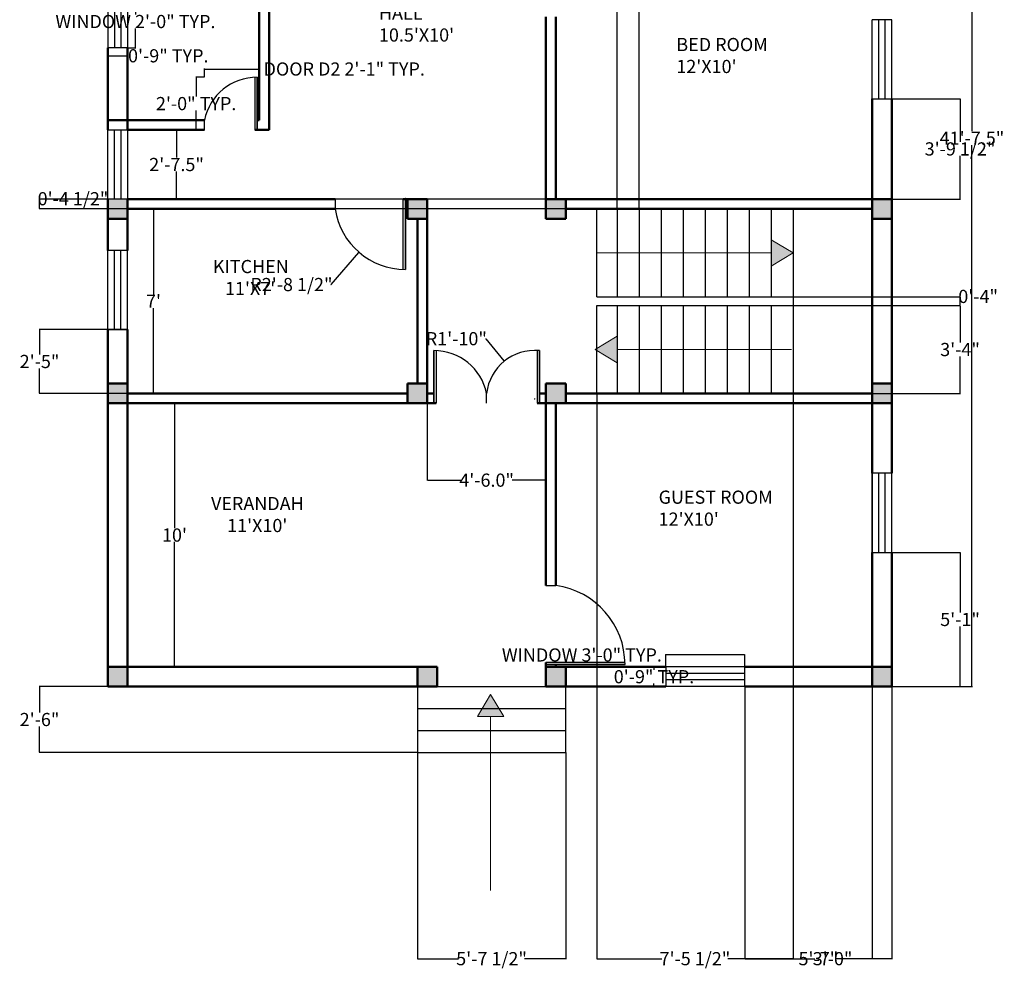
# Model space of a CAD drawing. Units: inches. Extents: x 1935 to 2390, y 6777 to 7449.
# Tile 1 of 2: x 1942 to 2390, y 6777 to 7213. Entities that reach past the tile are written whole.
import ezdxf

# ---------------------------------------------------------------- set-up
doc = ezdxf.new("R2010")
doc.units = ezdxf.units.IN
doc.header["$MEASUREMENT"] = 0
for name, color, linetype, lineweight in [('A-ANNO-DIMS', 7, 'Continuous', 18), ('A-ANNO-SYMB', 12, 'Continuous', 18), ('A-AREA-IDEN', 7, 'Continuous', 25), ('A-COLS', 42, 'Continuous', 50), ('A-COLS-PATT', 7, 'Continuous', 13), ('A-DOOR', 50, 'Continuous', 25), ('A-FLOR-STRS', 200, 'Continuous', 25), ('A-GLAZ', 140, 'Continuous', 25), ('A-WALL', 42, 'Continuous', 50)]:
    doc.layers.add(name, color=color, linetype=linetype, lineweight=lineweight)
doc.styles.get("Standard").update_dxf_attribs({"font": 'arial.ttf'})
doc.dimstyles.get("Standard").update_dxf_attribs({"dimtxt": 6, "dimasz": 0.18, "dimexe": 0.18, "dimexo": 0.0625, "dimgap": 0.09, "dimtad": 0, "dimtih": 1, "dimtoh": 1, "dimdec": 1, "dimzin": 0, "dimdsep": 46, "dimlunit": 3, "dimtxsty": 'Standard', "dimcen": 0.09, "dimclrd": 200, "dimclre": 200, "dimclrt": 200, "dimadec": 0, "dimazin": 0, "dimtfac": 1, "dimtdec": 1, "dimtofl": 0, "dimtmove": 0, "dimatfit": 3, "dimfxl": 1, "dimtolj": 1, "dimtzin": 0, "dimarcsym": 0})

# ---------------------------------------------------------------- blocks, each defined once
blk = doc.blocks.new('*D3')
at = {"layer": 'A-ANNO-DIMS', "color": 0, "lineweight": -2, "transparency": 16777216}
for p, q in [((1990.93, 7163.21), (2013.38, 7163.21)), ((2013.2, 7163.03), (2013.2, 7150.62)), ((2013.2, 7131.89), (2013.2, 7144.31)), ((1990.93, 7131.71), (2013.38, 7131.71))]:
    blk.add_line(p, q, dxfattribs=at)
at = {"layer": 'A-ANNO-DIMS', "color": 0, "transparency": 16777216}
for points in [[(2013.17, 7163.03), (2013.23, 7163.03), (2013.2, 7163.21)], [(2013.17, 7131.89), (2013.23, 7131.89), (2013.2, 7131.71)]]:
    blk.add_solid(points, dxfattribs=at)
at = {"layer": 'Defpoints', "color": 0, "transparency": 16777216}
for p in [(1990.87, 7163.21), (2013.2, 7163.21), (1990.87, 7131.71)]:
    blk.add_point(p, dxfattribs=at)
at = {"layer": 'A-ANNO-DIMS', "color": 0, "transparency": 16777216, "insert": (2013.2, 7147.46), "char_height": 6, "attachment_point": 5}
blk.add_mtext('\\A1;2\'-7.5"', dxfattribs=at)
blk = doc.blocks.new('*D4')
at = {"layer": 'A-ANNO-DIMS', "color": 0, "lineweight": -2, "transparency": 16777216}
for p, q in [((1990.93, 7127.21), (2002.86, 7127.21)), ((2002.68, 7127.03), (2002.68, 7088.3)), ((2002.68, 7043.39), (2002.68, 7082.12)), ((1990.93, 7043.21), (2002.86, 7043.21))]:
    blk.add_line(p, q, dxfattribs=at)
at = {"layer": 'A-ANNO-DIMS', "color": 0, "transparency": 16777216}
for points in [[(2002.65, 7127.03), (2002.71, 7127.03), (2002.68, 7127.21)], [(2002.65, 7043.39), (2002.71, 7043.39), (2002.68, 7043.21)]]:
    blk.add_solid(points, dxfattribs=at)
at = {"layer": 'Defpoints', "color": 0, "transparency": 16777216}
for p in [(1990.87, 7127.21), (1990.87, 7043.21), (2002.68, 7043.21)]:
    blk.add_point(p, dxfattribs=at)
at = {"layer": 'A-ANNO-DIMS', "color": 0, "transparency": 16777216, "insert": (2002.68, 7085.21), "char_height": 6, "attachment_point": 5}
blk.add_mtext("\\A1;7'", dxfattribs=at)
blk = doc.blocks.new('*D5')
at = {"layer": 'A-ANNO-DIMS', "color": 0, "lineweight": -2, "transparency": 16777216}
for p, q in [((1990.93, 7038.71), (2012.43, 7038.71)), ((2012.25, 7038.53), (2012.25, 6981.87)), ((2012.25, 6918.89), (2012.25, 6975.56)), ((1990.93, 6918.71), (2012.43, 6918.71))]:
    blk.add_line(p, q, dxfattribs=at)
at = {"layer": 'A-ANNO-DIMS', "color": 0, "transparency": 16777216}
for points in [[(2012.22, 7038.53), (2012.28, 7038.53), (2012.25, 7038.71)], [(2012.22, 6918.89), (2012.28, 6918.89), (2012.25, 6918.71)]]:
    blk.add_solid(points, dxfattribs=at)
at = {"layer": 'Defpoints', "color": 0, "transparency": 16777216}
for p in [(1990.87, 7038.71), (1990.87, 6918.71), (2012.25, 6918.71)]:
    blk.add_point(p, dxfattribs=at)
at = {"layer": 'A-ANNO-DIMS', "color": 0, "transparency": 16777216, "insert": (2012.25, 6978.71), "char_height": 6, "attachment_point": 5}
blk.add_mtext("\\A1;10'", dxfattribs=at)
blk = doc.blocks.new('*D6')
at = {"layer": 'A-ANNO-DIMS', "color": 0, "lineweight": -2, "transparency": 16777216}
for p, q in [((2127.37, 7038.65), (2127.37, 7003.54)), ((2181.37, 7038.65), (2181.37, 7003.54)), ((2127.55, 7003.72), (2142.68, 7003.72)), ((2181.19, 7003.72), (2166.05, 7003.72))]:
    blk.add_line(p, q, dxfattribs=at)
at = {"layer": 'A-ANNO-DIMS', "color": 0, "transparency": 16777216}
for points in [[(2127.55, 7003.75), (2127.55, 7003.69), (2127.37, 7003.72)], [(2181.19, 7003.75), (2181.19, 7003.69), (2181.37, 7003.72)]]:
    blk.add_solid(points, dxfattribs=at)
at = {"layer": 'Defpoints', "color": 0, "transparency": 16777216}
for p in [(2127.37, 7038.71), (2181.37, 7038.71), (2181.37, 7003.72)]:
    blk.add_point(p, dxfattribs=at)
at = {"layer": 'A-ANNO-DIMS', "color": 0, "transparency": 16777216, "insert": (2154.37, 7003.72), "char_height": 6, "attachment_point": 5}
blk.add_mtext('\\A1;4\'-6.0"', dxfattribs=at)
blk = doc.blocks.new('*D9')
at = {"layer": 'A-ANNO-DIMS', "color": 0, "lineweight": -2, "transparency": 16777216}
for p, q in [((2338.93, 7409.21), (2375.52, 7409.21)), ((2375.34, 7409.03), (2375.34, 7162.62)), ((2375.34, 6909.89), (2375.34, 7156.31)), ((2338.93, 6909.71), (2375.52, 6909.71))]:
    blk.add_line(p, q, dxfattribs=at)
at = {"layer": 'A-ANNO-DIMS', "color": 0, "transparency": 16777216}
for points in [[(2375.31, 7409.03), (2375.37, 7409.03), (2375.34, 7409.21)], [(2375.31, 6909.89), (2375.37, 6909.89), (2375.34, 6909.71)]]:
    blk.add_solid(points, dxfattribs=at)
at = {"layer": 'Defpoints', "color": 0, "transparency": 16777216}
for p in [(2338.87, 7409.21), (2338.87, 6909.71), (2375.34, 6909.71)]:
    blk.add_point(p, dxfattribs=at)
at = {"layer": 'A-ANNO-DIMS', "color": 0, "transparency": 16777216, "insert": (2375.34, 7159.46), "char_height": 6, "attachment_point": 5}
blk.add_mtext('\\A1;41\'-7.5"', dxfattribs=at)
blk = doc.blocks.new('WIN-36IN')
for p, q in [((0, 9), (0, 0)), ((0, 9), (36, 9)), ((36, 0), (36, 9)), ((0, 6), (36, 6)), ((0, 3), (36, 3)), ((0, 0), (36, 0))]:
    blk.add_line(p, q)
blk = doc.blocks.new('WIN-24IN')
for p, q in [((0, 24), (9, 24)), ((0, 24), (0, 0)), ((3, 24), (3, 0)), ((6, 24), (6, 0)), ((9, 24), (9, 0)), ((9, 0), (0, 0))]:
    blk.add_line(p, q)
blk = doc.blocks.new('DOOR-SINGLE-36IN')
for p, q in [((0, 37), (4.5, 37)), ((0, 1), (0, 2)), ((36, 2), (0, 2)), ((0, 0), (0, 1)), ((0, 1), (36, 1)), ((36, 1), (0, 1))]:
    blk.add_line(p, q)
blk.add_arc((-0.32, 1), 36.32, 0, 82.3719)
blk = doc.blocks.new('DOOR-SINGLE-24IN')
for p, q in [((23, 24), (23, 0)), ((24, 0), (24, 24)), ((24, 24), (24, 0)), ((0, 0), (0, 4.5)), ((24, 0), (23, 0)), ((25, 0), (24, 0))]:
    blk.add_line(p, q)
blk.add_arc((24, -0.52), 24.52, 90, 168.1877)
blk = doc.blocks.new('STAIR-DIRECTION')
h = blk.add_hatch(color=256)
h.dxf.hatch_style = 1
h.paths.add_polyline_path([(79.31, 12), (79.31, 0), (89.31, 6)])
for p, q in [((79.31, 12), (79.31, 0)), ((89.31, 6), (79.31, 12)), ((0, 6), (79.31, 6)), ((79.31, 0), (89.31, 6))]:
    blk.add_line(p, q)
blk = doc.blocks.new('*D16')
at = {"layer": 'A-ANNO-DIMS', "color": 200, "lineweight": -2, "transparency": 16777216}
for p, q in [((2235.96, 6924.11), (2235.78, 6924.11)), ((2235.96, 6918.78), (2235.96, 6924.29)), ((2271.78, 6924.11), (2236.14, 6924.11)), ((2271.96, 6918.78), (2271.96, 6924.29))]:
    blk.add_line(p, q, dxfattribs=at)
at = {"layer": 'A-ANNO-DIMS', "color": 200, "transparency": 16777216}
for points in [[(2236.14, 6924.14), (2236.14, 6924.08), (2235.96, 6924.11)], [(2271.78, 6924.14), (2271.78, 6924.08), (2271.96, 6924.11)]]:
    blk.add_solid(points, dxfattribs=at)
at = {"layer": 'Defpoints', "color": 0, "transparency": 16777216}
for p in [(2235.96, 6924.11), (2235.96, 6918.71), (2271.96, 6918.71)]:
    blk.add_point(p, dxfattribs=at)
at = {"layer": 'A-ANNO-DIMS', "color": 200, "transparency": 16777216, "insert": (2197.73, 6924.11), "char_height": 6, "attachment_point": 5}
blk.add_mtext('\\A1;WINDOW 3\'-0" TYP.', dxfattribs=at)
blk = doc.blocks.new('*D17')
at = {"layer": 'A-ANNO-DIMS', "color": 200, "lineweight": -2, "transparency": 16777216}
for p, q in [((2235.9, 6918.71), (2230.38, 6918.71)), ((2230.56, 6918.53), (2230.56, 6917.37)), ((2235.9, 6909.71), (2230.38, 6909.71)), ((2230.56, 6909.89), (2230.56, 6911.06))]:
    blk.add_line(p, q, dxfattribs=at)
at = {"layer": 'A-ANNO-DIMS', "color": 200, "transparency": 16777216}
for points in [[(2230.53, 6918.53), (2230.59, 6918.53), (2230.56, 6918.71)], [(2230.53, 6909.89), (2230.59, 6909.89), (2230.56, 6909.71)]]:
    blk.add_solid(points, dxfattribs=at)
at = {"layer": 'Defpoints', "color": 0, "transparency": 16777216}
for p in [(2235.96, 6918.71), (2230.56, 6909.71), (2235.96, 6909.71)]:
    blk.add_point(p, dxfattribs=at)
at = {"layer": 'A-ANNO-DIMS', "color": 200, "transparency": 16777216, "insert": (2230.56, 6914.21), "char_height": 6, "attachment_point": 5}
blk.add_mtext('\\A1;0\'-9" TYP.', dxfattribs=at)
blk = doc.blocks.new('*D18')
at = {"layer": 'A-ANNO-DIMS', "color": 200, "lineweight": -2, "transparency": 16777216}
for p, q in [((1990.93, 7224.58), (1994.65, 7224.58)), ((1994.47, 7224.4), (1994.47, 7215.77)), ((1994.47, 7200.76), (1994.47, 7209.39)), ((1990.93, 7200.58), (1994.65, 7200.58))]:
    blk.add_line(p, q, dxfattribs=at)
at = {"layer": 'A-ANNO-DIMS', "color": 200, "transparency": 16777216}
for points in [[(1994.44, 7224.4), (1994.5, 7224.4), (1994.47, 7224.58)], [(1994.44, 7200.76), (1994.5, 7200.76), (1994.47, 7200.58)]]:
    blk.add_solid(points, dxfattribs=at)
at = {"layer": 'Defpoints', "color": 0, "transparency": 16777216}
for p in [(1990.87, 7224.58), (1994.47, 7224.58), (1990.87, 7200.58)]:
    blk.add_point(p, dxfattribs=at)
at = {"layer": 'A-ANNO-DIMS', "color": 200, "transparency": 16777216, "insert": (1994.47, 7212.58), "char_height": 6, "attachment_point": 5}
blk.add_mtext('\\A1;WINDOW 2\'-0" TYP.', dxfattribs=at)
blk = doc.blocks.new('*D19')
at = {"layer": 'A-ANNO-DIMS', "color": 200, "lineweight": -2, "transparency": 16777216}
for p, q in [((1981.87, 7200.52), (1981.87, 7196.8)), ((1990.87, 7200.52), (1990.87, 7196.8)), ((1982.05, 7196.98), (1990.69, 7196.98)), ((1990.87, 7196.98), (1991.05, 7196.98))]:
    blk.add_line(p, q, dxfattribs=at)
at = {"layer": 'A-ANNO-DIMS', "color": 200, "transparency": 16777216}
for points in [[(1982.05, 7197.01), (1982.05, 7196.95), (1981.87, 7196.98)], [(1990.69, 7197.01), (1990.69, 7196.95), (1990.87, 7196.98)]]:
    blk.add_solid(points, dxfattribs=at)
at = {"layer": 'Defpoints', "color": 0, "transparency": 16777216}
for p in [(1981.87, 7200.58), (1990.87, 7200.58), (1990.87, 7196.98)]:
    blk.add_point(p, dxfattribs=at)
at = {"layer": 'A-ANNO-DIMS', "color": 200, "transparency": 16777216, "insert": (2009.42, 7196.98), "char_height": 6, "attachment_point": 5}
blk.add_mtext('\\A1;0\'-9" TYP.', dxfattribs=at)
blk = doc.blocks.new('*D22')
at = {"layer": 'A-ANNO-DIMS', "color": 200, "lineweight": -2, "transparency": 16777216}
for p, q in [((2025.87, 7187.28), (2025.87, 7191.14)), ((2026.05, 7190.96), (2050.69, 7190.96)), ((2050.87, 7187.28), (2050.87, 7191.14)), ((2050.87, 7190.96), (2051.05, 7190.96))]:
    blk.add_line(p, q, dxfattribs=at)
at = {"layer": 'A-ANNO-DIMS', "color": 200, "transparency": 16777216}
for points in [[(2026.05, 7190.99), (2026.05, 7190.93), (2025.87, 7190.96)], [(2050.69, 7190.99), (2050.69, 7190.93), (2050.87, 7190.96)]]:
    blk.add_solid(points, dxfattribs=at)
at = {"layer": 'Defpoints', "color": 0, "transparency": 16777216}
for p in [(2050.87, 7190.96), (2025.87, 7187.21), (2050.87, 7187.21)]:
    blk.add_point(p, dxfattribs=at)
at = {"layer": 'A-ANNO-DIMS', "color": 200, "transparency": 16777216, "insert": (2089.53, 7190.96), "char_height": 6, "attachment_point": 5}
blk.add_mtext('\\A1;DOOR D2 2\'-1" TYP.', dxfattribs=at)
blk = doc.blocks.new('*D23')
at = {"layer": 'A-ANNO-DIMS', "color": 200, "lineweight": -2, "transparency": 16777216}
for p, q in [((2025.8, 7187.21), (2021.94, 7187.21)), ((2022.12, 7187.03), (2022.12, 7178.37)), ((2022.12, 7163.39), (2022.12, 7172.06)), ((2025.8, 7163.21), (2021.94, 7163.21))]:
    blk.add_line(p, q, dxfattribs=at)
at = {"layer": 'A-ANNO-DIMS', "color": 200, "transparency": 16777216}
for points in [[(2022.09, 7187.03), (2022.15, 7187.03), (2022.12, 7187.21)], [(2022.09, 7163.39), (2022.15, 7163.39), (2022.12, 7163.21)]]:
    blk.add_solid(points, dxfattribs=at)
at = {"layer": 'Defpoints', "color": 0, "transparency": 16777216}
for p in [(2022.12, 7187.21), (2025.87, 7187.21), (2025.87, 7163.21)]:
    blk.add_point(p, dxfattribs=at)
at = {"layer": 'A-ANNO-DIMS', "color": 200, "transparency": 16777216, "insert": (2022.12, 7175.21), "char_height": 6, "attachment_point": 5}
blk.add_mtext('\\A1;2\'-0" TYP.', dxfattribs=at)
blk = doc.blocks.new('*D24')
at = {"layer": 'A-ANNO-DIMS', "color": 200, "lineweight": -2, "transparency": 16777216}
for p, q in [((2122.87, 6879.65), (2122.87, 6785.62)), ((2190.37, 6879.65), (2190.37, 6785.62)), ((2123.05, 6785.8), (2141.56, 6785.8)), ((2190.19, 6785.8), (2171.67, 6785.8))]:
    blk.add_line(p, q, dxfattribs=at)
at = {"layer": 'A-ANNO-DIMS', "color": 200, "transparency": 16777216}
for points in [[(2123.05, 6785.83), (2123.05, 6785.77), (2122.87, 6785.8)], [(2190.19, 6785.83), (2190.19, 6785.77), (2190.37, 6785.8)]]:
    blk.add_solid(points, dxfattribs=at)
at = {"layer": 'Defpoints', "color": 0, "transparency": 16777216}
for p in [(2122.87, 6879.71), (2190.37, 6879.71), (2190.37, 6785.8)]:
    blk.add_point(p, dxfattribs=at)
at = {"layer": 'A-ANNO-DIMS', "color": 200, "transparency": 16777216, "insert": (2156.62, 6785.8), "char_height": 6, "attachment_point": 5}
blk.add_mtext('\\A1;5\'-7 1/2"', dxfattribs=at)
blk = doc.blocks.new('*D25')
at = {"layer": 'A-ANNO-DIMS', "color": 200, "lineweight": -2, "transparency": 16777216}
for p, q in [((2122.8, 6909.71), (1950.64, 6909.71)), ((1950.82, 6909.53), (1950.82, 6897.87)), ((1950.82, 6879.89), (1950.82, 6891.56)), ((2122.8, 6879.71), (1950.64, 6879.71))]:
    blk.add_line(p, q, dxfattribs=at)
at = {"layer": 'A-ANNO-DIMS', "color": 200, "transparency": 16777216}
for points in [[(1950.79, 6909.53), (1950.85, 6909.53), (1950.82, 6909.71)], [(1950.79, 6879.89), (1950.85, 6879.89), (1950.82, 6879.71)]]:
    blk.add_solid(points, dxfattribs=at)
at = {"layer": 'Defpoints', "color": 0, "transparency": 16777216}
for p in [(1950.82, 6909.71), (2122.87, 6909.71), (2122.87, 6879.71)]:
    blk.add_point(p, dxfattribs=at)
at = {"layer": 'A-ANNO-DIMS', "color": 200, "transparency": 16777216, "insert": (1950.82, 6894.71), "char_height": 6, "attachment_point": 5}
blk.add_mtext('\\A1;2\'-6"', dxfattribs=at)
blk = doc.blocks.new('*D26')
at = {"layer": 'A-ANNO-DIMS', "color": 200, "lineweight": -2, "transparency": 16777216}
for p, q in [((2204.56, 7043.15), (2204.56, 6785.62)), ((2293.87, 7043.15), (2293.87, 6785.62)), ((2204.74, 6785.8), (2234.18, 6785.8)), ((2293.69, 6785.8), (2264.24, 6785.8))]:
    blk.add_line(p, q, dxfattribs=at)
at = {"layer": 'A-ANNO-DIMS', "color": 200, "transparency": 16777216}
for points in [[(2204.74, 6785.83), (2204.74, 6785.77), (2204.56, 6785.8)], [(2293.69, 6785.83), (2293.69, 6785.77), (2293.87, 6785.8)]]:
    blk.add_solid(points, dxfattribs=at)
at = {"layer": 'Defpoints', "color": 0, "transparency": 16777216}
for p in [(2204.56, 7043.21), (2293.87, 7043.21), (2293.87, 6785.8)]:
    blk.add_point(p, dxfattribs=at)
at = {"layer": 'A-ANNO-DIMS', "color": 200, "transparency": 16777216, "insert": (2249.21, 6785.8), "char_height": 6, "attachment_point": 5}
blk.add_mtext('\\A1;7\'-5 1/2"', dxfattribs=at)
blk = doc.blocks.new('*D27')
at = {"layer": 'A-ANNO-DIMS', "color": 200, "lineweight": -2, "transparency": 16777216}
for p, q in [((2293.93, 7083.21), (2370.1, 7083.21)), ((2369.92, 7083.03), (2369.92, 7066.37)), ((2369.92, 7043.39), (2369.92, 7060.06)), ((2293.93, 7043.21), (2370.1, 7043.21))]:
    blk.add_line(p, q, dxfattribs=at)
at = {"layer": 'A-ANNO-DIMS', "color": 200, "transparency": 16777216}
for points in [[(2369.89, 7083.03), (2369.95, 7083.03), (2369.92, 7083.21)], [(2369.89, 7043.39), (2369.95, 7043.39), (2369.92, 7043.21)]]:
    blk.add_solid(points, dxfattribs=at)
at = {"layer": 'Defpoints', "color": 0, "transparency": 16777216}
for p in [(2293.87, 7083.21), (2369.92, 7083.21), (2293.87, 7043.21)]:
    blk.add_point(p, dxfattribs=at)
at = {"layer": 'A-ANNO-DIMS', "color": 200, "transparency": 16777216, "insert": (2369.92, 7063.21), "char_height": 6, "attachment_point": 5}
blk.add_mtext('\\A1;3\'-4"', dxfattribs=at)
blk = doc.blocks.new('*D28')
at = {"layer": 'A-ANNO-DIMS', "color": 200, "lineweight": -2, "transparency": 16777216}
for p, q in [((2293.93, 7087.21), (2370.1, 7087.21)), ((2293.93, 7083.21), (2370.1, 7083.21)), ((2369.92, 7087.21), (2369.92, 7087.39)), ((2369.92, 7087.39), (2370.1, 7087.39)), ((2369.92, 7083.39), (2369.92, 7087.03))]:
    blk.add_line(p, q, dxfattribs=at)
at = {"layer": 'A-ANNO-DIMS', "color": 200, "transparency": 16777216}
for points in [[(2369.89, 7087.03), (2369.95, 7087.03), (2369.92, 7087.21)], [(2369.89, 7083.39), (2369.95, 7083.39), (2369.92, 7083.21)]]:
    blk.add_solid(points, dxfattribs=at)
at = {"layer": 'Defpoints', "color": 0, "transparency": 16777216}
for p in [(2293.87, 7087.21), (2293.87, 7083.21), (2369.92, 7087.21)]:
    blk.add_point(p, dxfattribs=at)
at = {"layer": 'A-ANNO-DIMS', "color": 200, "transparency": 16777216, "insert": (2378.16, 7087.39), "char_height": 6, "attachment_point": 5}
blk.add_mtext('\\A1;0\'-4"', dxfattribs=at)
blk = doc.blocks.new('*D29')
at = {"layer": 'A-ANNO-DIMS', "color": 200, "lineweight": -2, "transparency": 16777216}
for p, q in [((2293.87, 7043.15), (2293.87, 6785.62)), ((2329.87, 7043.15), (2329.87, 6785.62)), ((2294.05, 6785.8), (2303.8, 6785.8)), ((2329.69, 6785.8), (2319.93, 6785.8))]:
    blk.add_line(p, q, dxfattribs=at)
at = {"layer": 'A-ANNO-DIMS', "color": 200, "transparency": 16777216}
for points in [[(2294.05, 6785.83), (2294.05, 6785.77), (2293.87, 6785.8)], [(2329.69, 6785.83), (2329.69, 6785.77), (2329.87, 6785.8)]]:
    blk.add_solid(points, dxfattribs=at)
at = {"layer": 'Defpoints', "color": 0, "transparency": 16777216}
for p in [(2293.87, 7043.21), (2329.87, 7043.21), (2329.87, 6785.8)]:
    blk.add_point(p, dxfattribs=at)
at = {"layer": 'A-ANNO-DIMS', "color": 200, "transparency": 16777216, "insert": (2311.87, 6785.8), "char_height": 6, "attachment_point": 5}
blk.add_mtext('\\A1;3\'-0"', dxfattribs=at)
blk = doc.blocks.new('*D30')
at = {"layer": 'A-ANNO-DIMS', "color": 200, "lineweight": -2, "transparency": 16777216}
for p, q in [((2213.87, 7127.28), (2213.87, 7440.44)), ((2214.05, 7440.26), (2223.69, 7440.26)), ((2223.87, 7127.28), (2223.87, 7440.44)), ((2223.87, 7440.26), (2224.05, 7440.26))]:
    blk.add_line(p, q, dxfattribs=at)
at = {"layer": 'A-ANNO-DIMS', "color": 200, "transparency": 16777216}
for points in [[(2214.05, 7440.29), (2214.05, 7440.23), (2213.87, 7440.26)], [(2223.69, 7440.29), (2223.69, 7440.23), (2223.87, 7440.26)]]:
    blk.add_solid(points, dxfattribs=at)
at = {"layer": 'Defpoints', "color": 0, "transparency": 16777216}
for p in [(2223.87, 7440.26), (2213.87, 7127.21), (2223.87, 7127.21)]:
    blk.add_point(p, dxfattribs=at)
at = {"layer": 'A-ANNO-DIMS', "color": 200, "transparency": 16777216, "insert": (2234.44, 7440.26), "char_height": 6, "attachment_point": 5}
blk.add_mtext('\\A1;0\'-10"', dxfattribs=at)
blk = doc.blocks.new('*D31')
at = {"layer": 'A-ANNO-DIMS', "color": 200, "lineweight": -2, "transparency": 16777216}
for p, q in [((2181.3, 7131.71), (1950.64, 7131.71)), ((1950.82, 7131.71), (1950.82, 7131.89)), ((1950.82, 7131.89), (1951, 7131.89)), ((1950.82, 7127.39), (1950.82, 7131.53)), ((2190.3, 7127.21), (1950.64, 7127.21))]:
    blk.add_line(p, q, dxfattribs=at)
at = {"layer": 'A-ANNO-DIMS', "color": 200, "transparency": 16777216}
for points in [[(1950.79, 7131.53), (1950.85, 7131.53), (1950.82, 7131.71)], [(1950.79, 7127.39), (1950.85, 7127.39), (1950.82, 7127.21)]]:
    blk.add_solid(points, dxfattribs=at)
at = {"layer": 'Defpoints', "color": 0, "transparency": 16777216}
for p in [(1950.82, 7131.71), (2181.37, 7131.71), (2190.37, 7127.21)]:
    blk.add_point(p, dxfattribs=at)
at = {"layer": 'A-ANNO-DIMS', "color": 200, "transparency": 16777216, "insert": (1966.05, 7131.89), "char_height": 6, "attachment_point": 5}
blk.add_mtext('\\A1;0\'-4 1/2"', dxfattribs=at)
blk = doc.blocks.new('*D36')
at = {"layer": 'A-ANNO-DIMS', "color": 200, "lineweight": -2, "transparency": 16777216}
for p, q in [((2329.93, 7177.42), (2370.1, 7177.42)), ((2369.92, 7177.24), (2369.92, 7157.76)), ((2369.92, 7131.89), (2369.92, 7151.37)), ((2329.93, 7131.71), (2370.1, 7131.71))]:
    blk.add_line(p, q, dxfattribs=at)
at = {"layer": 'A-ANNO-DIMS', "color": 200, "transparency": 16777216}
for points in [[(2369.89, 7177.24), (2369.95, 7177.24), (2369.92, 7177.42)], [(2369.89, 7131.89), (2369.95, 7131.89), (2369.92, 7131.71)]]:
    blk.add_solid(points, dxfattribs=at)
at = {"layer": 'Defpoints', "color": 0, "transparency": 16777216}
for p in [(2329.87, 7177.42), (2369.92, 7177.42), (2329.87, 7131.71)]:
    blk.add_point(p, dxfattribs=at)
at = {"layer": 'A-ANNO-DIMS', "color": 200, "transparency": 16777216, "insert": (2369.92, 7154.57), "char_height": 6, "attachment_point": 5}
blk.add_mtext('\\A1;3\'-9 1/2"', dxfattribs=at)
blk = doc.blocks.new('*D37')
at = {"layer": 'A-ANNO-DIMS', "color": 200, "lineweight": -2, "transparency": 16777216}
for p, q in [((2338.93, 6970.84), (2370.1, 6970.84)), ((2369.92, 6970.66), (2369.92, 6943.43)), ((2369.92, 6909.89), (2369.92, 6937.12)), ((2338.93, 6909.71), (2370.1, 6909.71))]:
    blk.add_line(p, q, dxfattribs=at)
at = {"layer": 'A-ANNO-DIMS', "color": 200, "transparency": 16777216}
for points in [[(2369.89, 6970.66), (2369.95, 6970.66), (2369.92, 6970.84)], [(2369.89, 6909.89), (2369.95, 6909.89), (2369.92, 6909.71)]]:
    blk.add_solid(points, dxfattribs=at)
at = {"layer": 'Defpoints', "color": 0, "transparency": 16777216}
for p in [(2338.87, 6970.84), (2369.92, 6970.84), (2338.87, 6909.71)]:
    blk.add_point(p, dxfattribs=at)
at = {"layer": 'A-ANNO-DIMS', "color": 200, "transparency": 16777216, "insert": (2369.92, 6940.28), "char_height": 6, "attachment_point": 5}
blk.add_mtext('\\A1;5\'-1"', dxfattribs=at)
blk = doc.blocks.new('*D38')
at = {"layer": 'A-ANNO-DIMS', "color": 200, "lineweight": -2, "transparency": 16777216}
for p, q in [((2271.96, 6909.65), (2271.96, 6785.62)), ((2338.87, 6909.65), (2338.87, 6785.62)), ((2272.14, 6785.8), (2297.35, 6785.8)), ((2338.69, 6785.8), (2313.48, 6785.8))]:
    blk.add_line(p, q, dxfattribs=at)
at = {"layer": 'A-ANNO-DIMS', "color": 200, "transparency": 16777216}
for points in [[(2272.14, 6785.83), (2272.14, 6785.77), (2271.96, 6785.8)], [(2338.69, 6785.83), (2338.69, 6785.77), (2338.87, 6785.8)]]:
    blk.add_solid(points, dxfattribs=at)
at = {"layer": 'Defpoints', "color": 0, "transparency": 16777216}
for p in [(2271.96, 6909.71), (2338.87, 6909.71), (2338.87, 6785.8)]:
    blk.add_point(p, dxfattribs=at)
at = {"layer": 'A-ANNO-DIMS', "color": 200, "transparency": 16777216, "insert": (2305.41, 6785.8), "char_height": 6, "attachment_point": 5}
blk.add_mtext('\\A1;5\'-7"', dxfattribs=at)
blk = doc.blocks.new('*D41')
at = {"layer": 'A-ANNO-DIMS', "color": 200, "lineweight": -2, "transparency": 16777216}
for p, q in [((1990.8, 7072.32), (1950.64, 7072.32)), ((1950.82, 7072.14), (1950.82, 7060.92)), ((1950.82, 7043.39), (1950.82, 7054.62)), ((1990.8, 7043.21), (1950.64, 7043.21))]:
    blk.add_line(p, q, dxfattribs=at)
at = {"layer": 'A-ANNO-DIMS', "color": 200, "transparency": 16777216}
for points in [[(1950.79, 7072.14), (1950.85, 7072.14), (1950.82, 7072.32)], [(1950.79, 7043.39), (1950.85, 7043.39), (1950.82, 7043.21)]]:
    blk.add_solid(points, dxfattribs=at)
at = {"layer": 'Defpoints', "color": 0, "transparency": 16777216}
for p in [(1950.82, 7072.32), (1990.87, 7072.32), (1990.87, 7043.21)]:
    blk.add_point(p, dxfattribs=at)
at = {"layer": 'A-ANNO-DIMS', "color": 200, "transparency": 16777216, "insert": (1950.82, 7057.77), "char_height": 6, "attachment_point": 5}
blk.add_mtext('\\A1;2\'-5"', dxfattribs=at)
blk = doc.blocks.new('*D43')
at = {"layer": 'A-ANNO-DIMS', "color": 200, "lineweight": -2, "transparency": 16777216}
for p, q in [((2117.28, 7132.08), (2117.46, 7132.08)), ((2117.37, 7131.99), (2117.37, 7132.17)), ((2083.61, 7092.8), (2096.15, 7107.4)), ((2083.43, 7092.8), (2083.61, 7092.8))]:
    blk.add_line(p, q, dxfattribs=at)
at = {"layer": 'A-ANNO-DIMS', "color": 200, "transparency": 16777216}
blk.add_solid([(2096.13, 7107.42), (2096.17, 7107.38), (2096.27, 7107.53)], dxfattribs=at)
at = {"layer": 'Defpoints', "color": 0, "transparency": 16777216}
for p in [(2117.37, 7132.08), (2096.27, 7107.53)]:
    blk.add_point(p, dxfattribs=at)
at = {"layer": 'A-ANNO-DIMS', "color": 200, "transparency": 16777216, "insert": (2065.5, 7092.8), "char_height": 6, "attachment_point": 5}
blk.add_mtext('\\A1;R2\'-8 1/2"', dxfattribs=at)
blk = doc.blocks.new('*D45')
at = {"layer": 'A-ANNO-DIMS', "color": 200, "lineweight": -2, "transparency": 16777216}
for p, q in [((2153.85, 7068.15), (2154.03, 7068.15)), ((2154.03, 7068.15), (2162.26, 7058.01)), ((2176.2, 7040.75), (2176.38, 7040.75)), ((2176.29, 7040.66), (2176.29, 7040.84))]:
    blk.add_line(p, q, dxfattribs=at)
at = {"layer": 'A-ANNO-DIMS', "color": 200, "transparency": 16777216}
blk.add_solid([(2162.29, 7058.03), (2162.24, 7057.99), (2162.38, 7057.87)], dxfattribs=at)
at = {"layer": 'Defpoints', "color": 0, "transparency": 16777216}
for p in [(2162.38, 7057.87), (2176.29, 7040.75)]:
    blk.add_point(p, dxfattribs=at)
at = {"layer": 'A-ANNO-DIMS', "color": 200, "transparency": 16777216, "insert": (2140.58, 7068.15), "char_height": 6, "attachment_point": 5}
blk.add_mtext('\\A1;R1\'-10"', dxfattribs=at)

msp = doc.modelspace()

# ---------------------------------------------------------------- hatches: boundary and pattern name
at = {"layer": 'A-COLS-PATT'}
h = msp.add_hatch(color=256, dxfattribs=at)
h.dxf.hatch_style = 1
h.paths.add_polyline_path([(1990.87, 7409.21), (1981.87, 7409.21), (1981.87, 7400.21), (1990.87, 7400.21)])
h.paths.add_polyline_path([(2127.37, 7409.21), (2118.37, 7409.21), (2118.37, 7400.21), (2127.37, 7400.21)])
h.paths.add_polyline_path([(2190.37, 7409.21), (2181.37, 7409.21), (2181.37, 7400.21), (2190.37, 7400.21)])
h.paths.add_polyline_path([(2338.87, 7409.21), (2329.87, 7409.21), (2329.87, 7400.21), (2338.87, 7400.21)])
h.paths.add_polyline_path([(1990.87, 7260.71), (1981.87, 7260.71), (1981.87, 7251.71), (1990.87, 7251.71)])
h.paths.add_polyline_path([(2127.37, 7260.71), (2118.37, 7260.71), (2118.37, 7251.71), (2127.37, 7251.71)])
h.paths.add_polyline_path([(2190.37, 7260.71), (2181.37, 7260.71), (2181.37, 7251.71), (2190.37, 7251.71)])
h.paths.add_polyline_path([(2338.87, 7260.71), (2329.87, 7260.71), (2329.87, 7251.71), (2338.87, 7251.71)])
h.paths.add_polyline_path([(1990.87, 7131.71), (1981.87, 7131.71), (1981.87, 7122.71), (1990.87, 7122.71)])
h.paths.add_polyline_path([(2127.37, 7131.71), (2118.37, 7131.71), (2118.37, 7122.71), (2127.37, 7122.71)])
h.paths.add_polyline_path([(1990.87, 7047.71), (1981.87, 7047.71), (1981.87, 7038.71), (1990.87, 7038.71)])
h.paths.add_polyline_path([(2127.37, 7047.71), (2118.37, 7047.71), (2118.37, 7038.71), (2127.37, 7038.71)])
h.paths.add_polyline_path([(1990.87, 6918.71), (1981.87, 6918.71), (1981.87, 6909.71), (1990.87, 6909.71)])
h.paths.add_polyline_path([(2131.87, 6918.71), (2122.87, 6918.71), (2122.87, 6909.71), (2131.87, 6909.71)])
h.paths.add_polyline_path([(2190.37, 6918.71), (2181.37, 6918.71), (2181.37, 6909.71), (2190.37, 6909.71)])
h.paths.add_polyline_path([(2338.87, 6918.71), (2329.87, 6918.71), (2329.87, 6909.71), (2338.87, 6909.71)])
h.paths.add_polyline_path([(2190.37, 7047.71), (2181.37, 7047.71), (2181.37, 7038.71), (2190.37, 7038.71)])
h.paths.add_polyline_path([(2338.87, 7047.71), (2329.87, 7047.71), (2329.87, 7038.71), (2338.87, 7038.71)])
h.paths.add_polyline_path([(2190.37, 7131.71), (2181.37, 7131.71), (2181.37, 7122.71), (2190.37, 7122.71)])
h.paths.add_polyline_path([(2338.87, 7131.71), (2329.87, 7131.71), (2329.87, 7122.71), (2338.87, 7122.71)])

# ---------------------------------------------------------------- linework, layer by layer
at = {"layer": 'A-ANNO-SYMB'}
msp.add_line((2283.87, 7107.21), (2283.87, 7113.21), dxfattribs=at)
at = {"layer": 'A-COLS'}
for p, q in [((1981.87, 7131.71), (1981.87, 7122.71)), ((2127.37, 7131.71), (2118.37, 7131.71)), ((2118.37, 7131.71), (2118.37, 7122.71)), ((2181.37, 7131.71), (2190.37, 7131.71)), ((2181.37, 7122.71), (2181.37, 7131.71)), ((2190.37, 7131.71), (2190.37, 7122.71)), ((2329.87, 7131.71), (2329.87, 7122.71)), ((1981.87, 7122.71), (1990.87, 7122.71)), ((2118.37, 7122.71), (2127.37, 7122.71)), ((2190.37, 7122.71), (2181.37, 7122.71)), ((2329.87, 7122.71), (2338.87, 7122.71)), ((1981.87, 7038.71), (1981.87, 7047.71)), ((1981.87, 7047.71), (1990.87, 7047.71)), ((2127.37, 7047.71), (2118.37, 7047.71)), ((2118.37, 7047.71), (2118.37, 7038.71)), ((2127.37, 7038.71), (2127.37, 7047.71)), ((2181.37, 7038.71), (2181.37, 7047.71)), ((2181.37, 7047.71), (2190.37, 7047.71)), ((2190.37, 7047.71), (2190.37, 7038.71)), ((2338.87, 7047.71), (2329.87, 7047.71)), ((2329.87, 7047.71), (2329.87, 7038.71)), ((2338.87, 7038.71), (2338.87, 7047.71)), ((1981.87, 6909.71), (1981.87, 6918.71)), ((2122.87, 6918.71), (2122.87, 6909.71)), ((2122.87, 6918.71), (2131.87, 6918.71)), ((2131.87, 6918.71), (2131.87, 6909.71)), ((2181.37, 6918.71), (2190.37, 6918.71)), ((2190.37, 6918.71), (2190.37, 6909.71))]:
    msp.add_line(p, q, dxfattribs=at)
at = {"layer": 'A-DOOR'}
for p, q in [((2085.37, 7131.71), (2085.37, 7127.21)), ((2117.37, 7131.71), (2116.37, 7131.71)), ((2116.37, 7099.71), (2116.37, 7131.71)), ((2118.37, 7131.71), (2117.37, 7131.71)), ((2117.37, 7131.71), (2117.37, 7099.71)), ((2117.37, 7099.71), (2117.37, 7131.71)), ((2130.37, 7038.71), (2130.37, 7062.71)), ((2130.37, 7062.71), (2130.37, 7038.71)), ((2131.37, 7062.71), (2131.37, 7038.71)), ((2177.37, 7062.71), (2177.37, 7038.71)), ((2178.37, 7038.71), (2178.37, 7062.71)), ((2178.37, 7062.71), (2178.37, 7038.71)), ((2154.37, 7038.71), (2154.37, 7043.21)), ((2130.37, 7038.71), (2131.37, 7038.71)), ((2178.37, 7038.71), (2177.37, 7038.71)), ((2177.37, 7038.71), (2178.37, 7038.71))]:
    msp.add_line(p, q, dxfattribs=at)
for centre, radius, start, end in [((2117.37, 7132.08), 32.37, 188.6501, 270), ((2130.37, 7038.2), 24.52, 11.8123, 90), ((2176.29, 7040.75), 22.06, 84.5906, 173.5971)]:
    msp.add_arc(centre, radius, start, end, dxfattribs=at)
at = {"layer": 'A-FLOR-STRS'}
for p, q in [((2204.56, 7127.21), (2329.87, 7127.21)), ((2204.56, 7087.21), (2204.56, 7127.21)), ((2213.87, 7127.21), (2213.87, 7087.21)), ((2223.87, 7127.21), (2223.87, 7087.21)), ((2233.87, 7127.21), (2233.87, 7087.21)), ((2243.87, 7127.21), (2243.87, 7087.21)), ((2253.87, 7127.21), (2253.87, 7087.21)), ((2263.87, 7127.21), (2263.87, 7087.21)), ((2273.87, 7127.21), (2273.87, 7087.21)), ((2283.87, 7127.21), (2283.87, 7087.21)), ((2293.87, 7127.21), (2293.87, 7043.21)), ((2329.87, 7127.21), (2329.87, 7043.21)), ((2204.56, 7087.21), (2293.87, 7087.21)), ((2204.56, 7043.21), (2204.56, 7083.21)), ((2204.56, 7083.21), (2293.87, 7083.21)), ((2213.87, 7083.21), (2213.87, 7043.21)), ((2223.87, 7083.21), (2223.87, 7043.21)), ((2233.87, 7083.21), (2233.87, 7043.21)), ((2243.87, 7083.21), (2243.87, 7043.21)), ((2253.87, 7083.21), (2253.87, 7043.21)), ((2263.87, 7083.21), (2263.87, 7043.21)), ((2273.87, 7083.21), (2273.87, 7043.21)), ((2283.87, 7083.21), (2283.87, 7043.21)), ((2329.87, 7043.21), (2204.56, 7043.21)), ((2122.87, 6909.71), (2122.87, 6879.71)), ((2122.87, 6909.71), (2190.37, 6909.71)), ((2190.37, 6879.71), (2190.37, 6909.71)), ((2122.87, 6899.71), (2190.37, 6899.71)), ((2122.87, 6889.71), (2190.37, 6889.71)), ((2122.87, 6879.71), (2190.37, 6879.71))]:
    msp.add_line(p, q, dxfattribs=at)
at = {"layer": 'A-GLAZ'}
for p, q in [((1981.87, 7135.12), (1981.87, 7163.21)), ((1981.87, 7163.21), (1990.87, 7163.21)), ((1984.87, 7135.12), (1984.87, 7163.21)), ((1987.87, 7163.21), (1987.87, 7131.71)), ((1990.87, 7163.21), (1990.87, 7131.71)), ((1981.87, 7131.71), (1981.87, 7135.12)), ((1984.87, 7131.71), (1984.87, 7135.12)), ((1990.87, 7131.71), (1981.87, 7131.71))]:
    msp.add_line(p, q, dxfattribs=at)
at = {"layer": 'A-WALL'}
for p, q in [((2050.87, 7251.71), (2050.87, 7167.71)), ((2055.37, 7251.71), (2055.37, 7163.21)), ((2181.37, 7214.71), (2181.37, 7127.21)), ((2185.87, 7214.71), (2185.87, 7131.71)), ((1981.87, 7200.58), (1981.87, 7163.21)), ((1990.87, 7200.58), (1990.87, 7163.21)), ((2329.87, 7177.42), (2329.87, 7006.84)), ((2338.87, 7177.42), (2338.87, 7006.84)), ((1981.87, 7167.71), (2025.87, 7167.71)), ((2049.87, 7167.71), (2050.87, 7167.71)), ((1990.87, 7163.21), (2025.87, 7163.21)), ((2048.87, 7163.21), (2055.37, 7163.21)), ((1981.87, 7131.71), (1981.87, 7108.32)), ((1990.87, 7131.71), (2085.37, 7131.71)), ((1990.87, 7131.71), (1990.87, 7108.32)), ((2116.37, 7131.71), (2127.37, 7131.71)), ((2127.37, 7131.71), (2127.37, 7038.71)), ((2181.37, 7131.71), (2338.87, 7131.71)), ((2181.37, 7131.71), (2338.87, 7131.71)), ((1990.87, 7127.21), (2085.37, 7127.21)), ((2117.37, 7127.21), (2118.37, 7127.21)), ((2190.37, 7127.21), (2329.87, 7127.21)), ((2190.37, 7127.21), (2329.87, 7127.21)), ((2122.87, 7122.71), (2122.87, 7047.71)), ((1981.87, 7072.32), (1981.87, 6909.71)), ((1990.87, 7072.32), (1990.87, 6909.71)), ((1990.87, 7043.21), (2118.37, 7043.21)), ((2127.37, 7043.21), (2130.37, 7043.21)), ((2178.37, 7043.21), (2181.37, 7043.21)), ((2181.37, 7043.21), (2181.37, 6955.71)), ((2190.37, 7043.21), (2329.87, 7043.21)), ((2190.37, 7043.21), (2329.87, 7043.21)), ((1981.87, 7038.71), (2131.37, 7038.71)), ((2177.37, 7038.71), (2338.87, 7038.71)), ((2181.37, 7038.71), (2338.87, 7038.71)), ((2185.87, 7038.71), (2185.87, 6955.71)), ((2329.87, 6970.84), (2329.87, 6909.71)), ((2338.87, 6970.84), (2338.87, 6909.71)), ((1981.87, 6918.71), (2131.87, 6918.71)), ((2181.37, 6920.71), (2181.37, 6909.71)), ((2181.37, 6918.71), (2235.96, 6918.71)), ((2185.87, 6919.71), (2185.87, 6918.71)), ((2271.96, 6918.71), (2338.87, 6918.71)), ((1981.87, 6909.71), (2131.87, 6909.71)), ((2181.37, 6909.71), (2235.96, 6909.71)), ((2271.96, 6909.71), (2338.87, 6909.71))]:
    msp.add_line(p, q, dxfattribs=at)

# ---------------------------------------------------------------- block references
at = {"layer": 'A-ANNO-SYMB'}
msp.add_blockref('STAIR-DIRECTION', (2204.56, 7101.22), dxfattribs=at)
at = {"layer": 'A-ANNO-SYMB', "extrusion": (0, 0, -1), "zscale": -1}
msp.add_blockref('STAIR-DIRECTION', (-2293.17, 7057.22), dxfattribs=at)
at = {"layer": 'A-ANNO-SYMB', "extrusion": (0, 0, -1), "zscale": -1, "rotation": 90.00000000000207}
msp.add_blockref('STAIR-DIRECTION', (-2150.15, 6816.85), dxfattribs=at)
at = {"layer": 'A-DOOR'}
for name, p in [('DOOR-SINGLE-24IN', (2025.87, 7163.22)), ('DOOR-SINGLE-36IN', (2181.37, 6918.72))]:
    msp.add_blockref(name, p, dxfattribs=at)
at = {"layer": 'A-GLAZ'}
msp.add_blockref('WIN-24IN', (1981.87, 7200.58), dxfattribs=at)
for p, rotation in [((2338.87, 7177.42), 90.00000000000443), ((1990.87, 7072.32), 90.0000000000085), ((2338.87, 6970.84), 90.00000000000374), ((2271.96, 6918.71), 180)]:
    msp.add_blockref('WIN-36IN', p, dxfattribs=dict(at, rotation=rotation))

# ---------------------------------------------------------------- texts
at = {"layer": 'A-AREA-IDEN', "char_height": 6, "attachment_point": 1}
for s, width, insert in [("HALL\\P10.5'X10'", 47.0238, (2105.34, 7219.45)), ("BED ROOM\\P12'X10'", 55.6597, (2240.74, 7205.11)), ("KITCHEN\\P   11'X7'", 64.6607, (2029.75, 7104)), ("GUEST ROOM\\P12'X10'", 73.7986, (2232.68, 6998.97)), ("VERANDAH\\P    11'X10'", 87.9614, (2028.9, 6996.06))]:
    msp.add_mtext_dynamic_manual_height_columns(s, width=width, gutter_width=30, heights=[0], dxfattribs=dict(at, insert=insert))

# ---------------------------------------------------------------- dimensions: what is measured, and where the dimension line sits
at = {"layer": 'A-ANNO-DIMS'}
for base, p1, p2, override, picture, middle in [((2223.87, 7440.26), (2213.87, 7127.21), (2223.87, 7127.21), {"dimdec": 1, "dimlfac": 1, "dimrnd": 0, "dimzin": 1, "dimdsep": 46, "dimlunit": 4, "dimfrac": 2}, '*D30', (2234.44, 7440.26)), ((2293.87, 6785.8), (2204.56, 7043.21), (2293.87, 7043.21), {"dimdec": 1, "dimlfac": 1, "dimrnd": 0, "dimzin": 1, "dimdsep": 46, "dimlunit": 4, "dimfrac": 2}, '*D26', (2249.21, 6785.8)), ((2329.87, 6785.8), (2293.87, 7043.21), (2329.87, 7043.21), {"dimdec": 1, "dimlfac": 1, "dimrnd": 0, "dimzin": 1, "dimdsep": 46, "dimlunit": 4, "dimfrac": 2}, '*D29', (2311.87, 6785.8)), ((2181.37, 7003.72), (2127.37, 7038.71), (2181.37, 7038.71), {"dimclrd": 0, "dimclre": 0, "dimclrt": 0}, '*D6', (2154.37, 7003.72)), ((2338.87, 6785.8), (2271.96, 6909.71), (2338.87, 6909.71), {"dimdec": 1, "dimlfac": 1, "dimrnd": 0, "dimzin": 1, "dimdsep": 46, "dimlunit": 4, "dimfrac": 2}, '*D38', (2305.41, 6785.8)), ((2190.37, 6785.8), (2122.87, 6879.71), (2190.37, 6879.71), {"dimdec": 1, "dimlfac": 1, "dimrnd": 0, "dimzin": 1, "dimdsep": 46, "dimlunit": 4, "dimfrac": 2}, '*D24', (2156.62, 6785.8))]:
    dim = msp.add_linear_dim(base=base, p1=p1, p2=p2, dimstyle='Standard', override=override, dxfattribs=at)
    dim.commit()
    dim.dimension.update_dxf_attribs({"geometry": picture, "text_midpoint": middle})
for base, p1, p2, override, picture, middle in [((2375.34, 6909.71), (2338.87, 7409.21), (2338.87, 6909.71), {"dimclrd": 0, "dimclre": 0, "dimclrt": 0}, '*D9', (2375.34, 7159.46)), ((2369.92, 7177.42), (2329.87, 7131.71), (2329.87, 7177.42), {"dimdec": 1, "dimlfac": 1, "dimrnd": 0, "dimzin": 1, "dimdsep": 46, "dimlunit": 4, "dimfrac": 2}, '*D36', (2369.92, 7154.57)), ((2013.2, 7163.21), (1990.87, 7131.71), (1990.87, 7163.21), {"dimclrd": 0, "dimclre": 0, "dimclrt": 0}, '*D3', (2013.2, 7147.46)), ((1950.82, 7131.71), (2190.37, 7127.21), (2181.37, 7131.71), {"dimdec": 1, "dimlfac": 1, "dimrnd": 0, "dimzin": 1, "dimdsep": 46, "dimlunit": 4, "dimfrac": 2}, '*D31', (1966.05, 7131.89)), ((2002.68, 7043.21), (1990.87, 7127.21), (1990.87, 7043.21), {"dimclrd": 0, "dimclre": 0, "dimclrt": 0}, '*D4', (2002.68, 7085.21)), ((2369.92, 7087.21), (2293.87, 7083.21), (2293.87, 7087.21), {"dimdec": 1, "dimlfac": 1, "dimrnd": 0, "dimzin": 1, "dimdsep": 46, "dimlunit": 4, "dimfrac": 2}, '*D28', (2378.16, 7087.39)), ((2369.92, 7083.21), (2293.87, 7043.21), (2293.87, 7083.21), {"dimdec": 1, "dimlfac": 1, "dimrnd": 0, "dimzin": 1, "dimdsep": 46, "dimlunit": 4, "dimfrac": 2}, '*D27', (2369.92, 7063.21)), ((1950.82, 7072.32), (1990.87, 7043.21), (1990.87, 7072.32), {"dimdec": 1, "dimlfac": 1, "dimrnd": 0, "dimzin": 1, "dimdsep": 46, "dimlunit": 4, "dimfrac": 2}, '*D41', (1950.82, 7057.77)), ((2012.25, 6918.71), (1990.87, 7038.71), (1990.87, 6918.71), {"dimclrd": 0, "dimclre": 0, "dimclrt": 0}, '*D5', (2012.25, 6978.71)), ((2369.92, 6970.84), (2338.87, 6909.71), (2338.87, 6970.84), {"dimdec": 1, "dimlfac": 1, "dimrnd": 0, "dimzin": 1, "dimdsep": 46, "dimlunit": 4, "dimfrac": 2}, '*D37', (2369.92, 6940.28)), ((1950.82, 6909.71), (2122.87, 6879.71), (2122.87, 6909.71), {"dimdec": 1, "dimlfac": 1, "dimrnd": 0, "dimzin": 1, "dimdsep": 46, "dimlunit": 4, "dimfrac": 2}, '*D25', (1950.82, 6894.71))]:
    dim = msp.add_linear_dim(base=base, p1=p1, p2=p2, angle=90, dimstyle='Standard', override=override, dxfattribs=at)
    dim.commit()
    dim.dimension.update_dxf_attribs({"geometry": picture, "text_midpoint": middle})
for base, p1, p2, angle, text, picture, middle in [((1994.47, 7224.58), (1990.87, 7200.58), (1990.87, 7224.58), 90, 'WINDOW <> TYP.', '*D18', (1994.47, 7212.58)), ((2022.12, 7187.21), (2025.87, 7163.21), (2025.87, 7187.21), 90, '<> TYP.', '*D23', (2022.12, 7175.21)), ((2235.96, 6924.11), (2271.96, 6918.71), (2235.96, 6918.71), 180, 'WINDOW <> TYP.', '*D16', (2197.73, 6924.11)), ((2230.56, 6909.71), (2235.96, 6918.71), (2235.96, 6909.71), 270, '<> TYP.', '*D17', (2230.56, 6914.21))]:
    dim = msp.add_linear_dim(base=base, p1=p1, p2=p2, angle=angle, text=text, dimstyle='Standard', override={"dimdec": 1, "dimlfac": 1, "dimrnd": 0, "dimzin": 1, "dimdsep": 46, "dimlunit": 4, "dimfrac": 2}, dxfattribs=at)
    dim.commit()
    dim.dimension.update_dxf_attribs({"geometry": picture, "text_midpoint": middle})
for base, p1, p2, text, picture, middle in [((2050.87, 7190.96), (2025.87, 7187.21), (2050.87, 7187.21), 'DOOR D2 <> TYP.', '*D22', (2089.53, 7190.96)), ((1990.87, 7196.98), (1981.87, 7200.58), (1990.87, 7200.58), '<> TYP.', '*D19', (2009.42, 7196.98))]:
    dim = msp.add_linear_dim(base=base, p1=p1, p2=p2, text=text, dimstyle='Standard', override={"dimdec": 1, "dimlfac": 1, "dimrnd": 0, "dimzin": 1, "dimdsep": 46, "dimlunit": 4, "dimfrac": 2}, dxfattribs=at)
    dim.commit()
    dim.dimension.update_dxf_attribs({"geometry": picture, "text_midpoint": middle})
for center, mpoint, picture, middle in [((2117.37, 7132.08), (2096.27, 7107.53), '*D43', (2065.5, 7092.8)), ((2176.29, 7040.75), (2162.38, 7057.87), '*D45', (2140.58, 7068.15))]:
    dim = msp.add_radius_dim(center=center, mpoint=mpoint, dimstyle='Standard', override={"dimdec": 1, "dimlfac": 1, "dimrnd": 0, "dimzin": 1, "dimdsep": 46, "dimlunit": 4, "dimfrac": 2}, dxfattribs=at)
    dim.commit()
    dim.dimension.update_dxf_attribs({"geometry": picture, "text_midpoint": middle, "dimtype": 164})

doc.saveas('drawing.dxf')
